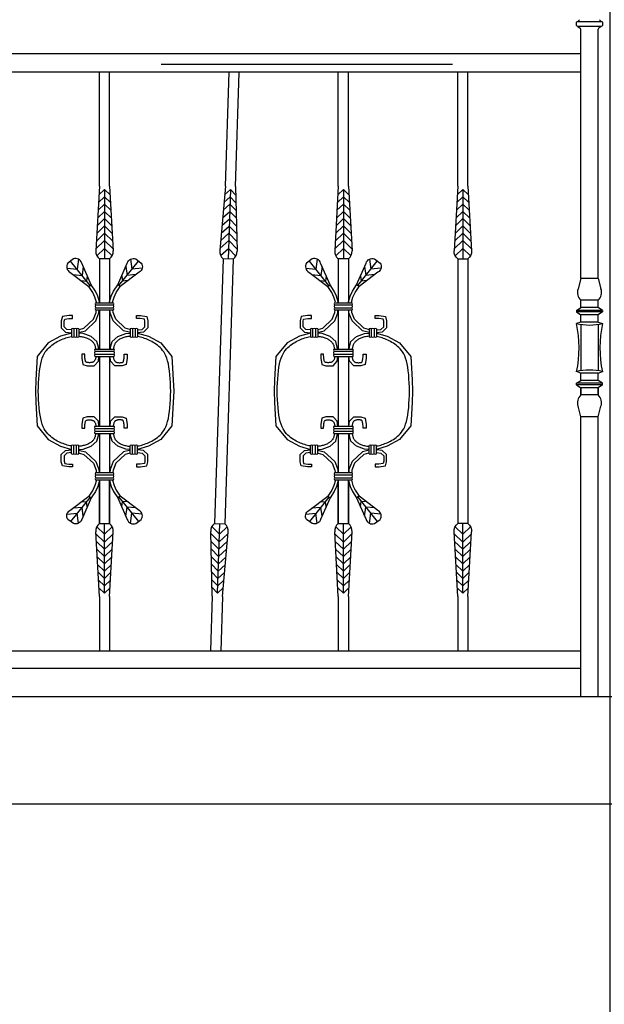
# Model space of a CAD drawing. Units: inches. Extents: x 2278 to 7495, y -71 to 1198.
# Tile 13 of 44: x 4938 to 4970, y 107 to 162. Entities that reach past the tile are written whole.
import ezdxf

# ---------------------------------------------------------------- set-up
doc = ezdxf.new("R2010")
doc.units = ezdxf.units.IN
doc.header["$MEASUREMENT"] = 0
doc.layers.add('A-ANNO-DIMS', color=2, linetype='Continuous', lineweight=18)
doc.layers.add('A-ELEV', color=7, linetype='Continuous', lineweight=25)
doc.styles.get("Standard").update_dxf_attribs({"font": 'arial.ttf'})
doc.dimstyles.get("Standard").update_dxf_attribs({"dimtxt": 6, "dimasz": 3, "dimexe": 0.18, "dimexo": 0.0625, "dimgap": 0.09, "dimtad": 0, "dimtih": 1, "dimtoh": 1, "dimdec": 0, "dimzin": 0, "dimdsep": 46, "dimlunit": 3, "dimtxsty": 'Standard', "dimblk": 'ARCHTICK', "dimcen": 0.09, "dimadec": 0, "dimazin": 0, "dimtfac": 1, "dimtdec": 0, "dimtofl": 0, "dimtmove": 0, "dimatfit": 3, "dimfxl": 1, "dimtolj": 1, "dimtzin": 0, "dimarcsym": 0})

# ---------------------------------------------------------------- blocks, each defined once
blk = doc.blocks.new('BALUSTER-ORNATE-C')
for p, q in [((3.585, 26.003), (3.585, 32.384)), ((4.155, 26.003), (4.155, 32.38)), ((3.585, 26.003), (3.383, 22.393)), ((4.155, 26.003), (4.357, 22.393)), ((3.533, 25.084), (3.87, 25.41)), ((3.557, 25.516), (3.87, 25.818)), ((3.87, 25.818), (3.87, 21.929)), ((4.182, 25.516), (3.87, 25.818)), ((4.206, 25.084), (3.87, 25.41)), ((3.509, 24.653), (3.87, 25.001)), ((4.231, 24.653), (3.87, 25.001)), ((3.485, 24.221), (3.87, 24.593)), ((4.255, 24.221), (3.87, 24.593)), ((3.437, 23.358), (3.87, 23.777)), ((3.461, 23.79), (3.87, 24.185)), ((4.279, 23.79), (3.87, 24.185)), ((4.303, 23.358), (3.87, 23.777)), ((3.412, 22.927), (3.87, 23.369)), ((4.327, 22.927), (3.87, 23.369)), ((3.388, 22.495), (3.87, 22.961)), ((4.351, 22.495), (3.87, 22.961)), ((3.441, 22.106), (3.87, 22.52)), ((4.298, 22.106), (3.87, 22.52)), ((3.063, 20.442), (1.97, 21.814)), ((2.412, 21.914), (2.338, 21.352)), ((2.678, 21.507), (2.613, 21.007)), ((3.585, 21.929), (3.585, 19.485)), ((4.155, 21.929), (3.585, 21.929)), ((4.155, 21.929), (4.155, 19.485)), ((4.677, 20.442), (5.769, 21.814)), ((5.061, 21.507), (5.127, 21.007)), ((5.328, 21.914), (5.401, 21.352)), ((1.774, 21.406), (2.338, 21.352)), ((2.111, 21.055), (2.613, 21.007)), ((2.907, 20.992), (2.867, 20.688)), ((4.833, 20.992), (4.872, 20.688)), ((5.629, 21.055), (5.127, 21.007)), ((5.966, 21.406), (5.401, 21.352)), ((2.562, 20.717), (2.867, 20.688)), ((5.177, 20.717), (4.872, 20.688)), ((3.37, 19.485), (4.37, 19.485)), ((3.37, 19.363), (4.37, 19.363)), ((3.37, 19.2), (4.37, 19.2)), ((3.37, 19.077), (4.37, 19.077)), ((3.585, 19.077), (3.585, 16.887)), ((4.155, 19.077), (4.155, 16.887)), ((2.026, 18.021), (2.026, 17.565)), ((2.148, 18.021), (2.148, 17.565)), ((2.311, 18.021), (2.311, 17.565)), ((2.433, 18.021), (2.433, 17.565)), ((5.306, 18.021), (5.306, 17.565)), ((5.428, 18.021), (5.428, 17.565)), ((5.591, 18.021), (5.591, 17.565)), ((5.714, 18.021), (5.714, 17.565)), ((3.329, 16.887), (4.411, 16.887)), ((3.329, 16.764), (4.411, 16.764)), ((3.329, 16.601), (4.411, 16.601)), ((3.329, 16.479), (4.411, 16.479)), ((3.585, 16.479), (3.585, 12.578)), ((4.155, 16.479), (4.155, 12.578)), ((3.329, 12.578), (4.411, 12.578)), ((3.329, 12.456), (4.411, 12.456)), ((3.329, 12.293), (4.411, 12.293)), ((3.329, 12.171), (4.411, 12.171)), ((3.585, 12.171), (3.585, 9.98)), ((4.155, 12.171), (4.155, 9.98)), ((2.026, 11.037), (2.026, 11.493)), ((2.148, 11.037), (2.148, 11.493)), ((2.311, 11.037), (2.311, 11.493)), ((2.433, 11.037), (2.433, 11.493)), ((5.306, 11.037), (5.306, 11.493)), ((5.428, 11.037), (5.428, 11.493)), ((5.591, 11.037), (5.591, 11.493)), ((5.714, 11.037), (5.714, 11.493)), ((3.37, 9.98), (4.37, 9.98)), ((3.37, 9.858), (4.37, 9.858)), ((3.37, 9.695), (4.37, 9.695)), ((3.37, 9.573), (4.37, 9.573)), ((3.585, 9.573), (3.585, 7.095)), ((3.585, 7.095), (3.585, 9.573)), ((4.155, 9.573), (4.155, 7.095)), ((4.155, 7.095), (4.155, 9.573)), ((3.063, 8.615), (1.97, 7.244)), ((2.562, 8.34), (2.867, 8.37)), ((2.907, 8.066), (2.867, 8.37)), ((4.677, 8.615), (5.769, 7.244)), ((4.833, 8.066), (4.872, 8.37)), ((5.177, 8.34), (4.872, 8.37)), ((2.111, 8.002), (2.613, 8.051)), ((2.678, 7.551), (2.613, 8.051)), ((5.061, 7.551), (5.127, 8.051)), ((5.629, 8.002), (5.127, 8.051)), ((1.774, 7.651), (2.338, 7.706)), ((2.412, 7.143), (2.338, 7.706)), ((5.328, 7.143), (5.401, 7.706)), ((5.966, 7.651), (5.401, 7.706)), ((3.585, 3.055), (3.383, 6.664)), ((3.441, 6.952), (3.87, 6.538)), ((3.585, 7.128), (4.155, 7.128)), ((3.87, 3.24), (3.87, 7.128)), ((4.298, 6.952), (3.87, 6.538)), ((4.155, 3.055), (4.357, 6.664)), ((3.388, 6.562), (3.87, 6.097)), ((3.412, 6.131), (3.87, 5.689)), ((4.351, 6.562), (3.87, 6.097)), ((4.327, 6.131), (3.87, 5.689)), ((3.437, 5.699), (3.87, 5.28)), ((4.303, 5.699), (3.87, 5.28)), ((3.461, 5.268), (3.87, 4.872)), ((4.279, 5.268), (3.87, 4.872)), ((3.485, 4.836), (3.87, 4.464)), ((4.255, 4.836), (3.87, 4.464)), ((3.509, 4.405), (3.87, 4.056)), ((3.533, 3.973), (3.87, 3.648)), ((4.231, 4.405), (3.87, 4.056)), ((4.206, 3.973), (3.87, 3.648)), ((3.557, 3.542), (3.87, 3.24)), ((4.182, 3.542), (3.87, 3.24)), ((3.585, 3.055), (3.585, 0)), ((4.155, 3.055), (4.155, 0))]:
    blk.add_line(p, q)
for points in [[(3.131, 20.487), (2.594, 21.696, 0.435351), (2.128, 21.929), (1.813, 21.699, 0.435351), (1.936, 21.192), (2.995, 20.398)], [(4.608, 20.487), (5.145, 21.696, -0.435351), (5.612, 21.929), (5.927, 21.699, -0.435351), (5.804, 21.192), (4.745, 20.398)], [(3.131, 8.571), (2.594, 7.362, -0.435351), (2.128, 7.128), (1.813, 7.359, -0.435351), (1.936, 7.866), (2.995, 8.66)], [(4.608, 8.571), (5.145, 7.362, 0.435351), (5.612, 7.128), (5.927, 7.359, 0.435351), (5.804, 7.866), (4.745, 8.66)]]:
    blk.add_lwpolyline(points, format="xyb", close=True)
for points in [[(3.42, 19.485), (3.421, 19.506), (3.336, 19.795), (3.216, 20.057), (2.995, 20.398)], [(3.583, 19.485), (3.585, 19.526), (3.489, 19.852), (3.359, 20.135), (3.131, 20.487)], [(4.157, 19.485), (4.155, 19.526), (4.25, 19.852), (4.38, 20.135), (4.608, 20.487)], [(4.32, 19.485), (4.319, 19.506), (4.403, 19.795), (4.523, 20.057), (4.745, 20.398)], [(2.026, 17.961), (1.767, 17.989), (1.612, 18.138), (1.612, 18.447), (1.642, 18.56), (1.879, 18.596), (2.084, 18.596), (2.084, 18.759), (1.866, 18.759), (1.512, 18.705), (1.449, 18.469), (1.449, 18.069), (1.694, 17.833), (2.026, 17.797)], [(2.433, 17.826), (2.492, 17.833), (2.801, 17.915), (3.385, 18.463), (3.557, 18.908), (3.565, 19.077)], [(2.433, 17.99), (2.462, 17.993), (2.719, 18.062), (3.247, 18.557), (3.396, 18.942), (3.402, 19.077)], [(5.306, 17.826), (5.247, 17.833), (4.939, 17.915), (4.355, 18.463), (4.182, 18.908), (4.175, 19.077)], [(5.306, 17.99), (5.278, 17.993), (5.02, 18.062), (4.493, 18.557), (4.344, 18.942), (4.338, 19.077)], [(5.714, 17.961), (5.973, 17.989), (6.128, 18.138), (6.128, 18.447), (6.098, 18.56), (5.861, 18.596), (5.656, 18.596), (5.656, 18.759), (5.873, 18.759), (6.227, 18.705), (6.291, 18.469), (6.291, 18.069), (6.046, 17.833), (5.714, 17.797)], [(2.026, 17.782), (1.412, 17.603), (0.722, 17.231), (0.095, 16.469), (0.025, 15.162), (0, 14.529), (0.025, 13.895), (0.095, 12.589), (0.722, 11.827), (1.412, 11.455), (2.026, 11.276)], [(3.541, 16.887), (3.527, 17.004), (3.446, 17.313), (3.128, 17.594), (2.683, 17.766), (2.433, 17.777)], [(4.198, 16.887), (4.212, 17.004), (4.294, 17.313), (4.612, 17.594), (5.057, 17.766), (5.306, 17.777)], [(5.714, 17.782), (6.328, 17.603), (7.018, 17.231), (7.644, 16.469), (7.715, 15.162), (7.74, 14.529), (7.715, 13.895), (7.644, 12.589), (7.018, 11.827), (6.328, 11.455), (5.714, 11.276)], [(0.163, 14.522), (0.173, 14.759), (0.184, 14.995), (0.199, 15.227), (0.217, 15.452), (0.239, 15.667), (0.267, 15.87), (0.3, 16.057), (0.34, 16.227), (0.386, 16.376), (0.438, 16.508), (0.495, 16.624), (0.557, 16.727), (0.623, 16.819), (0.692, 16.9), (0.764, 16.975), (0.839, 17.043), (0.916, 17.105), (0.993, 17.163), (1.071, 17.216), (1.15, 17.265), (1.229, 17.309), (1.309, 17.35), (1.389, 17.388), (1.469, 17.422), (1.548, 17.454), (1.627, 17.484), (1.705, 17.51), (1.782, 17.533), (1.858, 17.553), (1.933, 17.571), (2.007, 17.585), (2.026, 17.587)], [(2.433, 17.606), (2.499, 17.6), (2.563, 17.592), (2.624, 17.582), (2.683, 17.57), (2.739, 17.556), (2.792, 17.54), (2.842, 17.522), (2.891, 17.503), (2.937, 17.482), (2.981, 17.46), (3.023, 17.436), (3.064, 17.41), (3.102, 17.384), (3.138, 17.357), (3.171, 17.329), (3.201, 17.301), (3.228, 17.272), (3.251, 17.244), (3.271, 17.217), (3.288, 17.19), (3.303, 17.162), (3.316, 17.134), (3.327, 17.104), (3.337, 17.072), (3.345, 17.038), (3.354, 17.001), (3.361, 16.962), (3.368, 16.922), (3.374, 16.887)], [(5.306, 17.606), (5.241, 17.6), (5.177, 17.592), (5.115, 17.582), (5.057, 17.57), (5.001, 17.556), (4.948, 17.54), (4.897, 17.522), (4.849, 17.503), (4.803, 17.482), (4.759, 17.46), (4.716, 17.436), (4.676, 17.41), (4.638, 17.384), (4.602, 17.357), (4.569, 17.329), (4.539, 17.301), (4.512, 17.272), (4.488, 17.244), (4.468, 17.217), (4.451, 17.19), (4.437, 17.162), (4.424, 17.134), (4.413, 17.104), (4.403, 17.072), (4.394, 17.038), (4.386, 17.001), (4.379, 16.962), (4.371, 16.922), (4.366, 16.887)], [(7.577, 14.522), (7.567, 14.759), (7.555, 14.995), (7.541, 15.227), (7.523, 15.452), (7.501, 15.667), (7.473, 15.87), (7.44, 16.057), (7.4, 16.227), (7.354, 16.376), (7.302, 16.508), (7.244, 16.624), (7.183, 16.727), (7.117, 16.819), (7.048, 16.9), (6.976, 16.975), (6.901, 17.043), (6.824, 17.105), (6.747, 17.163), (6.668, 17.216), (6.59, 17.265), (6.51, 17.309), (6.431, 17.35), (6.351, 17.388), (6.271, 17.422), (6.191, 17.454), (6.113, 17.484), (6.035, 17.51), (5.958, 17.533), (5.882, 17.553), (5.807, 17.571), (5.733, 17.585), (5.714, 17.587)], [(3.388, 16.479), (3.383, 16.441), (3.376, 16.401), (3.368, 16.364), (3.357, 16.329), (3.346, 16.299), (3.333, 16.271), (3.318, 16.247), (3.303, 16.225), (3.286, 16.207), (3.268, 16.19), (3.249, 16.176), (3.228, 16.164), (3.205, 16.154), (3.179, 16.145), (3.149, 16.138), (3.116, 16.133), (3.081, 16.13), (3.045, 16.129), (3.007, 16.129), (2.971, 16.131), (2.936, 16.134), (2.905, 16.137), (2.88, 16.142), (2.863, 16.146), (2.852, 16.151), (2.845, 16.154), (2.84, 16.159), (2.834, 16.166), (2.825, 16.18), (2.814, 16.203), (2.803, 16.237), (2.792, 16.28), (2.783, 16.331), (2.775, 16.388), (2.769, 16.452), (2.766, 16.522), (2.764, 16.599), (2.601, 16.596), (2.601, 16.378), (2.656, 16.024), (2.892, 15.961), (3.291, 15.961), (3.527, 16.206), (3.557, 16.479)], [(4.352, 16.479), (4.357, 16.441), (4.364, 16.401), (4.372, 16.364), (4.382, 16.329), (4.394, 16.299), (4.407, 16.271), (4.421, 16.247), (4.437, 16.225), (4.454, 16.207), (4.472, 16.19), (4.491, 16.176), (4.512, 16.164), (4.534, 16.154), (4.56, 16.145), (4.59, 16.138), (4.623, 16.133), (4.659, 16.13), (4.695, 16.129), (4.732, 16.129), (4.769, 16.131), (4.804, 16.134), (4.835, 16.137), (4.86, 16.142), (4.877, 16.146), (4.888, 16.151), (4.894, 16.154), (4.899, 16.159), (4.906, 16.166), (4.914, 16.18), (4.925, 16.203), (4.937, 16.237), (4.948, 16.28), (4.957, 16.331), (4.965, 16.388), (4.971, 16.452), (4.974, 16.522), (4.975, 16.599), (5.138, 16.596), (5.138, 16.378), (5.084, 16.024), (4.848, 15.961), (4.448, 15.961), (4.212, 16.206), (4.182, 16.479)], [(2.026, 11.47), (2.007, 11.473), (1.933, 11.487), (1.858, 11.504), (1.782, 11.524), (1.705, 11.548), (1.627, 11.574), (1.548, 11.603), (1.469, 11.635), (1.389, 11.67), (1.309, 11.708), (1.229, 11.748), (1.15, 11.793), (1.071, 11.841), (0.993, 11.894), (0.916, 11.952), (0.839, 12.015), (0.764, 12.083), (0.692, 12.157), (0.623, 12.239), (0.557, 12.33), (0.495, 12.433), (0.438, 12.549), (0.386, 12.681), (0.34, 12.831), (0.3, 13), (0.267, 13.188), (0.239, 13.391), (0.217, 13.606), (0.199, 13.831), (0.184, 14.062), (0.173, 14.298), (0.163, 14.536)], [(5.714, 11.47), (5.733, 11.473), (5.807, 11.487), (5.882, 11.504), (5.958, 11.524), (6.035, 11.548), (6.113, 11.574), (6.191, 11.603), (6.271, 11.635), (6.351, 11.67), (6.431, 11.708), (6.51, 11.748), (6.59, 11.793), (6.668, 11.841), (6.747, 11.894), (6.824, 11.952), (6.901, 12.015), (6.976, 12.083), (7.048, 12.157), (7.117, 12.239), (7.183, 12.33), (7.244, 12.433), (7.302, 12.549), (7.354, 12.681), (7.4, 12.831), (7.44, 13), (7.473, 13.188), (7.501, 13.391), (7.523, 13.606), (7.541, 13.831), (7.555, 14.062), (7.567, 14.298), (7.577, 14.536)], [(3.557, 12.578), (3.527, 12.852), (3.291, 13.097), (2.892, 13.097), (2.656, 13.033), (2.601, 12.679), (2.601, 12.462), (2.764, 12.459), (2.766, 12.536), (2.769, 12.605), (2.775, 12.669), (2.783, 12.727), (2.792, 12.778), (2.803, 12.82), (2.814, 12.854), (2.825, 12.878), (2.834, 12.892), (2.84, 12.899), (2.845, 12.903), (2.852, 12.907), (2.863, 12.911), (2.88, 12.916), (2.905, 12.92), (2.936, 12.924), (2.971, 12.927), (3.007, 12.929), (3.045, 12.929), (3.081, 12.928), (3.116, 12.924), (3.149, 12.919), (3.179, 12.912), (3.205, 12.904), (3.228, 12.893), (3.249, 12.881), (3.268, 12.867), (3.286, 12.851), (3.303, 12.832), (3.318, 12.811), (3.333, 12.786), (3.346, 12.759), (3.357, 12.728), (3.368, 12.694), (3.376, 12.656), (3.383, 12.616), (3.388, 12.578)], [(4.182, 12.578), (4.212, 12.852), (4.448, 13.097), (4.848, 13.097), (5.084, 13.033), (5.138, 12.679), (5.138, 12.462), (4.975, 12.459), (4.974, 12.536), (4.971, 12.605), (4.965, 12.669), (4.957, 12.727), (4.948, 12.778), (4.937, 12.82), (4.925, 12.854), (4.914, 12.878), (4.906, 12.892), (4.899, 12.899), (4.894, 12.903), (4.888, 12.907), (4.877, 12.911), (4.86, 12.916), (4.835, 12.92), (4.804, 12.924), (4.769, 12.927), (4.732, 12.929), (4.695, 12.929), (4.659, 12.928), (4.623, 12.924), (4.59, 12.919), (4.56, 12.912), (4.534, 12.904), (4.512, 12.893), (4.491, 12.881), (4.472, 12.867), (4.454, 12.851), (4.437, 12.832), (4.421, 12.811), (4.407, 12.786), (4.394, 12.759), (4.382, 12.728), (4.372, 12.694), (4.364, 12.656), (4.357, 12.616), (4.352, 12.578)], [(3.374, 12.171), (3.368, 12.136), (3.361, 12.095), (3.354, 12.056), (3.345, 12.02), (3.337, 11.986), (3.327, 11.954), (3.316, 11.924), (3.303, 11.895), (3.288, 11.868), (3.271, 11.841), (3.251, 11.813), (3.228, 11.785), (3.201, 11.757), (3.171, 11.729), (3.138, 11.701), (3.102, 11.673), (3.064, 11.647), (3.023, 11.622), (2.981, 11.598), (2.937, 11.576), (2.891, 11.555), (2.842, 11.535), (2.792, 11.518), (2.739, 11.502), (2.683, 11.488), (2.624, 11.476), (2.563, 11.465), (2.499, 11.457), (2.433, 11.451)], [(2.433, 11.28), (2.683, 11.291), (3.128, 11.464), (3.446, 11.745), (3.527, 12.053), (3.541, 12.171)], [(5.306, 11.28), (5.057, 11.291), (4.612, 11.464), (4.294, 11.745), (4.212, 12.053), (4.198, 12.171)], [(4.366, 12.171), (4.371, 12.136), (4.379, 12.095), (4.386, 12.056), (4.394, 12.02), (4.403, 11.986), (4.413, 11.954), (4.424, 11.924), (4.437, 11.895), (4.451, 11.868), (4.468, 11.841), (4.488, 11.813), (4.512, 11.785), (4.539, 11.757), (4.569, 11.729), (4.602, 11.701), (4.638, 11.673), (4.676, 11.647), (4.716, 11.622), (4.759, 11.598), (4.803, 11.576), (4.849, 11.555), (4.897, 11.535), (4.948, 11.518), (5.001, 11.502), (5.057, 11.488), (5.115, 11.476), (5.177, 11.465), (5.241, 11.457), (5.306, 11.451)], [(2.026, 11.097), (1.767, 11.069), (1.612, 10.919), (1.612, 10.611), (1.642, 10.498), (1.879, 10.461), (2.084, 10.461), (2.084, 10.298), (1.866, 10.298), (1.512, 10.353), (1.449, 10.589), (1.449, 10.988), (1.694, 11.225), (2.026, 11.261)], [(2.433, 11.232), (2.492, 11.225), (2.801, 11.143), (3.385, 10.594), (3.557, 10.149), (3.565, 9.98)], [(2.433, 11.067), (2.462, 11.064), (2.719, 10.996), (3.247, 10.501), (3.396, 10.115), (3.402, 9.98)], [(5.306, 11.232), (5.247, 11.225), (4.939, 11.143), (4.355, 10.594), (4.182, 10.149), (4.175, 9.98)], [(5.306, 11.067), (5.278, 11.064), (5.02, 10.996), (4.493, 10.501), (4.344, 10.115), (4.338, 9.98)], [(5.714, 11.097), (5.973, 11.069), (6.128, 10.919), (6.128, 10.611), (6.098, 10.498), (5.861, 10.461), (5.656, 10.461), (5.656, 10.298), (5.873, 10.298), (6.227, 10.353), (6.291, 10.589), (6.291, 10.988), (6.046, 11.225), (5.714, 11.261)], [(3.42, 9.573), (3.421, 9.552), (3.336, 9.262), (3.216, 9.001), (2.995, 8.66)], [(3.583, 9.573), (3.585, 9.532), (3.489, 9.205), (3.359, 8.922), (3.131, 8.571)], [(4.157, 9.573), (4.155, 9.532), (4.25, 9.205), (4.38, 8.922), (4.608, 8.571)], [(4.32, 9.573), (4.319, 9.552), (4.403, 9.262), (4.523, 9.001), (4.745, 8.66)]]:
    blk.add_lwpolyline(points)
for centre, radius, start, end in [((3.929, 22.355), 0.547, 176.0178, 231.0717), ((3.811, 22.355), 0.547, 308.9283, 3.9822), ((3.475, 19.424), 0.121, 149.7768, 210.2232), ((3.563, 19.281), 0.209, 157.1017, 202.8983), ((4.265, 19.424), 0.121, 329.7768, 30.2232), ((4.177, 19.281), 0.209, 337.1017, 22.8983), ((3.475, 19.139), 0.121, 149.7768, 210.2232), ((4.265, 19.139), 0.121, 329.7768, 30.2232), ((2.087, 17.916), 0.121, 59.7768, 120.2232), ((2.23, 17.828), 0.209, 67.1017, 112.8983), ((2.372, 17.916), 0.121, 59.7768, 120.2232), ((5.367, 17.916), 0.121, 59.7768, 120.2232), ((5.51, 17.828), 0.209, 67.1017, 112.8983), ((5.653, 17.916), 0.121, 59.7768, 120.2232), ((2.087, 17.67), 0.121, 239.7768, 300.2232), ((2.23, 17.758), 0.209, 247.1017, 292.8983), ((2.372, 17.67), 0.121, 239.7768, 300.2232), ((5.367, 17.67), 0.121, 239.7768, 300.2232), ((5.51, 17.758), 0.209, 247.1017, 292.8983), ((5.653, 17.67), 0.121, 239.7768, 300.2232), ((3.434, 16.825), 0.121, 149.7768, 210.2232), ((3.522, 16.683), 0.209, 157.1017, 202.8983), ((3.434, 16.54), 0.121, 149.7768, 210.2232), ((4.306, 16.825), 0.121, 329.7768, 30.2232), ((4.218, 16.683), 0.209, 337.1017, 22.8983), ((4.306, 16.54), 0.121, 329.7768, 30.2232), ((3.434, 12.517), 0.121, 149.7768, 210.2232), ((3.522, 12.375), 0.209, 157.1017, 202.8983), ((3.434, 12.232), 0.121, 149.7768, 210.2232), ((4.306, 12.517), 0.121, 329.7768, 30.2232), ((4.218, 12.375), 0.209, 337.1017, 22.8983), ((4.306, 12.232), 0.121, 329.7768, 30.2232), ((2.087, 11.388), 0.121, 59.7768, 120.2232), ((2.087, 11.142), 0.121, 239.7768, 300.2232), ((2.23, 11.3), 0.209, 67.1017, 112.8983), ((2.23, 11.23), 0.209, 247.1017, 292.8983), ((2.372, 11.388), 0.121, 59.7768, 120.2232), ((2.372, 11.142), 0.121, 239.7768, 300.2232), ((5.367, 11.388), 0.121, 59.7768, 120.2232), ((5.367, 11.142), 0.121, 239.7768, 300.2232), ((5.51, 11.3), 0.209, 67.1017, 112.8983), ((5.51, 11.23), 0.209, 247.1017, 292.8983), ((5.653, 11.388), 0.121, 59.7768, 120.2232), ((5.653, 11.142), 0.121, 239.7768, 300.2232), ((3.475, 9.919), 0.121, 149.7768, 210.2232), ((4.265, 9.919), 0.121, 329.7768, 30.2232), ((3.563, 9.776), 0.209, 157.1017, 202.8983), ((3.475, 9.634), 0.121, 149.7768, 210.2232), ((4.177, 9.776), 0.209, 337.1017, 22.8983), ((4.265, 9.634), 0.121, 329.7768, 30.2232), ((3.929, 6.703), 0.547, 128.9283, 183.9822), ((3.811, 6.703), 0.547, 356.0178, 51.0717)]:
    blk.add_arc(centre, radius, start, end)
blk = doc.blocks.new('RAIL-BAR-A')
for p, q in [((0.202, 26.003), (0.202, 32.38)), ((0.773, 26.003), (0.773, 32.38)), ((0.202, 26.003), (0, 22.393)), ((0.773, 26.003), (0.975, 22.393)), ((0.151, 25.084), (0.488, 25.41)), ((0.175, 25.516), (0.488, 25.818)), ((0.488, 25.818), (0.488, 21.929)), ((0.8, 25.516), (0.488, 25.818)), ((0.824, 25.084), (0.488, 25.41)), ((0.127, 24.653), (0.488, 25.001)), ((0.848, 24.653), (0.488, 25.001)), ((0.103, 24.221), (0.488, 24.593)), ((0.873, 24.221), (0.488, 24.593)), ((0.054, 23.358), (0.488, 23.777)), ((0.079, 23.79), (0.488, 24.185)), ((0.897, 23.79), (0.488, 24.185)), ((0.921, 23.358), (0.488, 23.777)), ((0.03, 22.927), (0.488, 23.369)), ((0.945, 22.927), (0.488, 23.369)), ((0.006, 22.495), (0.488, 22.961)), ((0.969, 22.495), (0.488, 22.961)), ((0.059, 22.106), (0.488, 22.52)), ((0.916, 22.106), (0.488, 22.52)), ((0.202, 21.929), (0.202, 7.128)), ((0.773, 21.929), (0.202, 21.929)), ((0.773, 21.929), (0.773, 7.128)), ((0.202, 3.055), (0, 6.664)), ((0.059, 6.952), (0.488, 6.538)), ((0.202, 7.128), (0.773, 7.128)), ((0.488, 3.24), (0.488, 7.128)), ((0.916, 6.952), (0.488, 6.538)), ((0.773, 3.055), (0.975, 6.664)), ((0.006, 6.562), (0.488, 6.097)), ((0.03, 6.131), (0.488, 5.689)), ((0.969, 6.562), (0.488, 6.097)), ((0.945, 6.131), (0.488, 5.689)), ((0.054, 5.699), (0.488, 5.28)), ((0.921, 5.699), (0.488, 5.28)), ((0.079, 5.268), (0.488, 4.872)), ((0.897, 5.268), (0.488, 4.872)), ((0.103, 4.836), (0.488, 4.464)), ((0.873, 4.836), (0.488, 4.464)), ((0.127, 4.405), (0.488, 4.056)), ((0.151, 3.973), (0.488, 3.648)), ((0.848, 4.405), (0.488, 4.056)), ((0.824, 3.973), (0.488, 3.648)), ((0.175, 3.542), (0.488, 3.24)), ((0.8, 3.542), (0.488, 3.24)), ((0.202, 3.055), (0.202, 0)), ((0.773, 3.055), (0.773, 0))]:
    blk.add_line(p, q)
for centre, start, end in [((0.546, 22.355), 176.0178, 231.0717), ((0.429, 22.355), 308.9283, 3.9822), ((0.546, 6.703), 128.9283, 183.9822), ((0.429, 6.703), 356.0178, 51.0717)]:
    blk.add_arc(centre, 0.547, start, end)
blk = doc.blocks.new('RAIL-BAR-B')
for p, q in [((17.353, 32.832), (1.059, 32.832)), ((0.203, 26.003), (0.203, 32.38)), ((0.773, 26.003), (0.773, 32.38)), ((0.203, 26.003), (0.001, 22.393)), ((0.773, 26.003), (0.976, 22.393)), ((0.152, 25.084), (0.488, 25.41)), ((0.176, 25.516), (0.488, 25.818)), ((0.488, 25.818), (0.488, 21.929)), ((0.801, 25.516), (0.488, 25.818)), ((0.825, 25.084), (0.488, 25.41)), ((0.128, 24.653), (0.488, 25.001)), ((0.849, 24.653), (0.488, 25.001)), ((0.103, 24.221), (0.488, 24.593)), ((0.873, 24.221), (0.488, 24.593)), ((0.055, 23.358), (0.488, 23.777)), ((0.079, 23.79), (0.488, 24.185)), ((0.897, 23.79), (0.488, 24.185)), ((0.922, 23.358), (0.488, 23.777)), ((0.031, 22.927), (0.488, 23.369)), ((0.946, 22.927), (0.488, 23.369)), ((0.007, 22.495), (0.488, 22.961)), ((0.97, 22.495), (0.488, 22.961)), ((0.06, 22.106), (0.488, 22.52)), ((0.917, 22.106), (0.488, 22.52)), ((0.203, 21.929), (0.203, 7.128)), ((0.773, 21.929), (0.203, 21.929)), ((0.773, 21.929), (0.773, 7.128)), ((0.203, 3.055), (0.001, 6.664)), ((0.06, 6.952), (0.488, 6.538)), ((0.203, 7.128), (0.773, 7.128)), ((0.488, 3.24), (0.488, 7.128)), ((0.917, 6.952), (0.488, 6.538)), ((0.773, 3.055), (0.976, 6.664)), ((0.007, 6.562), (0.488, 6.097)), ((0.031, 6.131), (0.488, 5.689)), ((0.97, 6.562), (0.488, 6.097)), ((0.946, 6.131), (0.488, 5.689)), ((0.055, 5.699), (0.488, 5.28)), ((0.922, 5.699), (0.488, 5.28)), ((0.079, 5.268), (0.488, 4.872)), ((0.897, 5.268), (0.488, 4.872)), ((0.103, 4.836), (0.488, 4.464)), ((0.873, 4.836), (0.488, 4.464)), ((0.128, 4.405), (0.488, 4.056)), ((0.152, 3.973), (0.488, 3.648)), ((0.849, 4.405), (0.488, 4.056)), ((0.825, 3.973), (0.488, 3.648)), ((0.176, 3.542), (0.488, 3.24)), ((0.801, 3.542), (0.488, 3.24)), ((0.203, 3.055), (0.203, 0)), ((0.773, 3.055), (0.773, 0))]:
    blk.add_line(p, q)
for centre, start, end in [((0.547, 22.355), 176.0178, 231.0717), ((0.429, 22.355), 308.9283, 3.9822), ((0.547, 6.703), 128.9283, 183.9822), ((0.429, 6.703), 356.0178, 51.0717)]:
    blk.add_arc(centre, 0.547, start, end)
blk = doc.blocks.new('_ArchTick')
at = {"color": 0, "linetype": 'ByBlock', "const_width": 0.15}
blk.add_lwpolyline([(-0.5, -0.5), (0.5, 0.5)], dxfattribs=at)
blk = doc.blocks.new('*D123')
at = {"layer": 'A-ANNO-DIMS', "color": 0, "lineweight": -2, "transparency": 16777216}
for p, q in [((4736.95, 340.157), (4736.95, -23.427)), ((5145.676, -1.81), (5145.676, -23.427)), ((4736.95, -23.247), (4923.929, -23.247)), ((5145.676, -23.247), (4958.697, -23.247))]:
    blk.add_line(p, q, dxfattribs=at)
at = {"layer": 'Defpoints', "color": 0, "transparency": 16777216}
for p in [(4736.95, 340.219), (5145.676, -1.747), (5145.676, -23.247)]:
    blk.add_point(p, dxfattribs=at)
at = {"layer": 'A-ANNO-DIMS', "color": 0, "lineweight": -2, "transparency": 16777216, "xscale": 3, "yscale": 3, "zscale": 3, "rotation": 180}
blk.add_blockref('_ArchTick', (4736.95, -23.247), dxfattribs=at)
at = {"layer": 'A-ANNO-DIMS', "color": 0, "lineweight": -2, "transparency": 16777216, "xscale": 3, "yscale": 3, "zscale": 3}
blk.add_blockref('_ArchTick', (5145.676, -23.247), dxfattribs=at)
at = {"layer": 'A-ANNO-DIMS', "color": 0, "transparency": 16777216, "insert": (4941.313, -23.247), "char_height": 6, "attachment_point": 5}
blk.add_mtext('\\A1;34\'-0 1/2"', dxfattribs=at)
blk = doc.blocks.new('*D128')
at = {"layer": 'A-ANNO-DIMS', "color": 0, "lineweight": -2, "transparency": 16777216}
for p, q in [((4909.676, 99.315), (4909.676, 361.899)), ((4970.676, 60.779), (4970.676, 361.899)), ((4909.676, 361.719), (4932.111, 361.719)), ((4970.676, 361.719), (4948.241, 361.719))]:
    blk.add_line(p, q, dxfattribs=at)
at = {"layer": 'Defpoints', "color": 0, "transparency": 16777216}
for p in [(4970.676, 361.719), (4909.676, 99.253), (4970.676, 60.717)]:
    blk.add_point(p, dxfattribs=at)
at = {"layer": 'A-ANNO-DIMS', "color": 0, "lineweight": -2, "transparency": 16777216, "xscale": 3, "yscale": 3, "zscale": 3, "rotation": 180}
blk.add_blockref('_ArchTick', (4909.676, 361.719), dxfattribs=at)
at = {"layer": 'A-ANNO-DIMS', "color": 0, "lineweight": -2, "transparency": 16777216, "xscale": 3, "yscale": 3, "zscale": 3}
blk.add_blockref('_ArchTick', (4970.676, 361.719), dxfattribs=at)
at = {"layer": 'A-ANNO-DIMS', "color": 0, "transparency": 16777216, "insert": (4940.176, 361.719), "char_height": 6, "attachment_point": 5}
blk.add_mtext('\\A1;5\'-1"', dxfattribs=at)
blk = doc.blocks.new('*D129')
at = {"layer": 'A-ANNO-DIMS', "color": 0, "lineweight": -2, "transparency": 16777216}
for p, q in [((4970.676, 60.779), (4970.676, 361.899)), ((5016.176, 99.315), (5016.176, 361.899)), ((4970.676, 361.719), (4978.373, 361.719)), ((5016.176, 361.719), (5008.479, 361.719))]:
    blk.add_line(p, q, dxfattribs=at)
at = {"layer": 'Defpoints', "color": 0, "transparency": 16777216}
for p in [(5016.176, 361.719), (5016.176, 99.253), (4970.676, 60.717)]:
    blk.add_point(p, dxfattribs=at)
at = {"layer": 'A-ANNO-DIMS', "color": 0, "lineweight": -2, "transparency": 16777216, "xscale": 3, "yscale": 3, "zscale": 3, "rotation": 180}
blk.add_blockref('_ArchTick', (4970.676, 361.719), dxfattribs=at)
at = {"layer": 'A-ANNO-DIMS', "color": 0, "lineweight": -2, "transparency": 16777216, "xscale": 3, "yscale": 3, "zscale": 3}
blk.add_blockref('_ArchTick', (5016.176, 361.719), dxfattribs=at)
at = {"layer": 'A-ANNO-DIMS', "color": 0, "transparency": 16777216, "insert": (4993.426, 361.719), "char_height": 6, "attachment_point": 5}
blk.add_mtext('\\A1;3\'-9 1/2"', dxfattribs=at)

msp = doc.modelspace()

# ---------------------------------------------------------------- linework, layer by layer
at = {"layer": 'A-ELEV'}
for p, q in [((4968.876, 162.015), (4968.962, 162.112)), ((4970.179, 162.015), (4970.093, 162.112)), ((4968.876, 161.735), (4969.009, 161.64)), ((4969.039, 147.642), (4969.039, 161.577)), ((4970.016, 147.642), (4970.016, 161.577)), ((4970.179, 161.735), (4970.046, 161.64)), ((4969.039, 160.198), (4875.673, 160.198)), ((4969.039, 159.179), (4875.673, 159.179)), ((4969.039, 147.642), (4968.886, 147.049)), ((4970.016, 147.642), (4969.039, 147.642)), ((4970.016, 147.642), (4970.169, 147.049)), ((4968.794, 145.849), (4969.039, 146.012)), ((4970.016, 146.42), (4969.039, 146.42)), ((4969.039, 146.012), (4969.039, 146.42)), ((4970.016, 146.012), (4969.039, 146.012)), ((4970.016, 146.012), (4970.016, 146.42)), ((4970.261, 145.849), (4970.016, 146.012)), ((4968.794, 145.849), (4968.794, 145.768)), ((4970.261, 145.849), (4968.794, 145.849)), ((4968.794, 145.768), (4969.039, 145.605)), ((4970.261, 145.768), (4968.794, 145.768)), ((4970.016, 145.605), (4969.039, 145.605)), ((4969.039, 145.198), (4969.039, 145.605)), ((4970.261, 145.768), (4970.016, 145.605)), ((4970.016, 145.198), (4970.016, 145.605)), ((4970.261, 145.849), (4970.261, 145.768)), ((4969.039, 145.198), (4968.794, 145.116)), ((4970.016, 145.198), (4969.039, 145.198)), ((4969.039, 145.07), (4969.039, 142.474)), ((4970.016, 145.198), (4970.261, 145.116)), ((4970.016, 145.07), (4970.016, 142.474)), ((4969.039, 142.346), (4968.794, 142.428)), ((4969.039, 141.936), (4969.039, 142.346)), ((4970.016, 142.346), (4969.039, 142.346)), ((4970.016, 142.346), (4970.261, 142.428)), ((4970.016, 141.936), (4970.016, 142.346)), ((4968.794, 141.773), (4969.039, 141.936)), ((4968.794, 141.691), (4968.794, 141.773)), ((4970.261, 141.773), (4968.794, 141.773)), ((4968.794, 141.691), (4969.039, 141.529)), ((4970.261, 141.691), (4968.794, 141.691)), ((4970.016, 141.936), (4969.039, 141.936)), ((4970.261, 141.773), (4970.016, 141.936)), ((4970.261, 141.691), (4970.016, 141.529)), ((4970.261, 141.691), (4970.261, 141.773)), ((4969.039, 141.529), (4969.039, 141.121)), ((4969.039, 141.121), (4969.039, 141.529)), ((4970.016, 141.529), (4969.039, 141.529)), ((4970.016, 141.121), (4969.039, 141.121)), ((4970.016, 141.529), (4970.016, 141.121)), ((4970.016, 141.121), (4970.016, 141.529)), ((4969.039, 139.899), (4968.886, 140.492)), ((4970.016, 139.899), (4970.169, 140.492)), ((4970.016, 139.899), (4969.039, 139.899)), ((4969.039, 124.253), (4969.039, 139.899)), ((4970.016, 124.253), (4970.016, 139.899)), ((4969.039, 126.799), (4875.673, 126.799)), ((4969.039, 125.821), (4875.673, 125.821)), ((4874.676, 124.253), (5145.676, 124.253)), ((4874.676, 118.253), (5145.676, 118.253))]:
    msp.add_line(p, q, dxfattribs=at)
msp.add_lwpolyline([(4970.179, 161.735), (4968.876, 161.735, -0.414214), (4968.794, 161.816), (4968.794, 161.934, -0.414214), (4968.876, 162.015), (4970.179, 162.015, -0.414214), (4970.261, 161.934), (4970.261, 161.816, -0.414214)], format="xyb", close=True, dxfattribs=at)
for centre, radius, start, end in [((4968.957, 161.577), 0.0815, 0, 50.672), ((4970.098, 161.577), 0.0815, 129.328, 180), ((4969.462, 146.856), 0.608, 161.4732, 225.8681), ((4969.593, 146.856), 0.608, 314.1319, 18.5268), ((4969.527, 148.339), 3.305, 257.1818, 282.8182), ((4962.424, 143.743), 6.517, 348.3176, 12.1601), ((4976.631, 143.743), 6.517, 167.8399, 191.6824), ((4969.527, 139.205), 3.305, 77.1818, 102.8182), ((4969.462, 140.685), 0.608, 134.1319, 198.5268), ((4969.593, 140.685), 0.608, 341.4732, 45.8681)]:
    msp.add_arc(centre, radius, start, end, dxfattribs=at)

# ---------------------------------------------------------------- block references
for p in [(4938.528, 126.799), (4951.889, 126.799)]:
    msp.add_blockref('BALUSTER-ORNATE-C', p, dxfattribs=at)
at = {"layer": 'A-ELEV', "extrusion": (0, 0, -1), "zscale": -1}
msp.add_blockref('RAIL-BAR-B', (-4962.928, 126.799), dxfattribs=at)
at = {"layer": 'A-ELEV', "rotation": 358.1636620689618}
msp.add_blockref('RAIL-BAR-A', (4948.123, 126.822), dxfattribs=at)

# ---------------------------------------------------------------- dimensions: what is measured, and where the dimension line sits
at = {"layer": 'A-ANNO-DIMS'}
for base, p1, p2, picture, middle in [((5016.176, 361.719), (4970.676, 60.717), (5016.176, 99.253), '*D129', (4993.426, 361.719)), ((4970.676, 361.719), (4909.676, 99.253), (4970.676, 60.717), '*D128', (4940.176, 361.719)), ((5145.676, -23.247), (4736.95, 340.219), (5145.676, -1.747), '*D123', (4941.313, -23.247))]:
    dim = msp.add_linear_dim(base=base, p1=p1, p2=p2, dimstyle='Standard', override={"dimdec": 1, "dimlfac": 1, "dimrnd": 0, "dimzin": 1, "dimdsep": 46, "dimlunit": 4, "dimfrac": 2}, dxfattribs=at)
    dim.commit()
    dim.dimension.update_dxf_attribs({"geometry": picture, "text_midpoint": middle})

doc.saveas('drawing.dxf')
